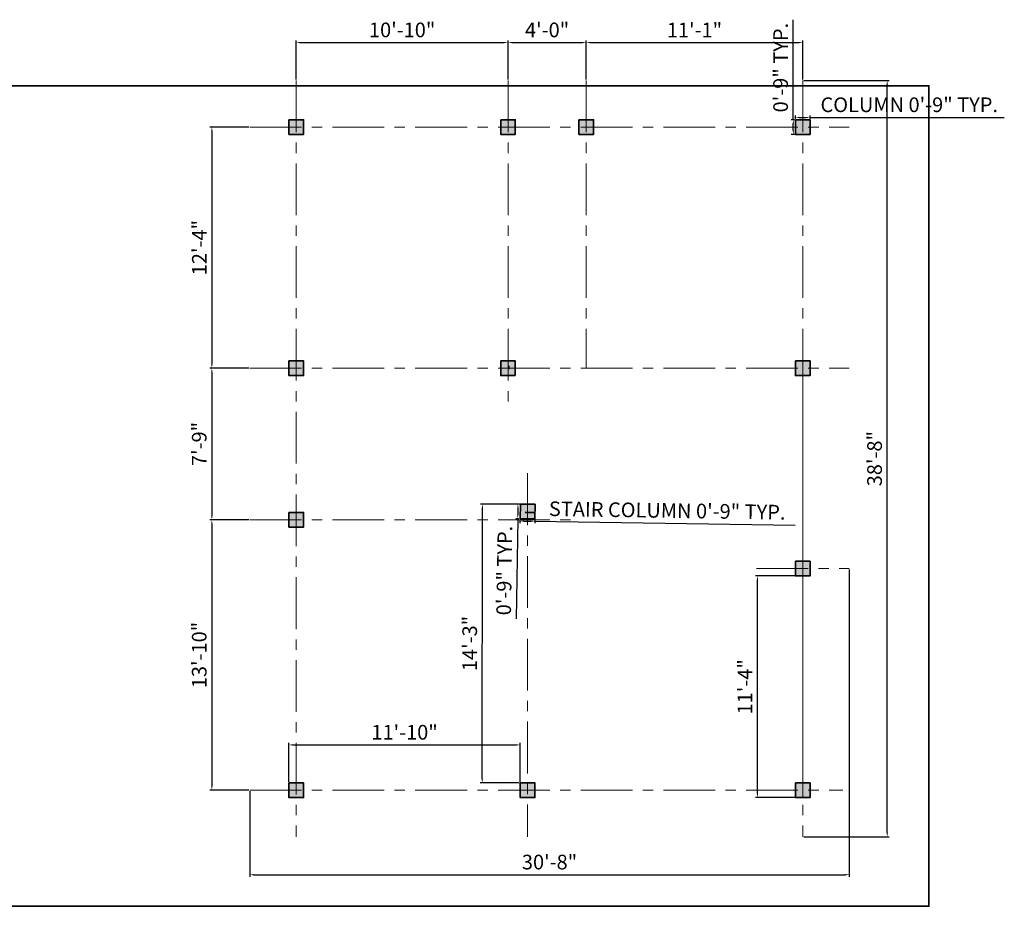
# Model space of a CAD drawing. Units: inches. Extents: x 2289 to 3796, y 1741 to 2286.
# Tile 4 of 4: x 3192 to 3796, y 1742 to 2286. Entities that reach past the tile are written whole.
import ezdxf

# ---------------------------------------------------------------- set-up
doc = ezdxf.new("R2010")
doc.units = ezdxf.units.IN
doc.linetypes.add('CENTER', pattern=[50.8, 31.75, -6.35, 6.35, -6.35])
for name, color, linetype, lineweight in [('A-ANNO-DIMS', 2, 'Continuous', 18), ('A-ANNO-TTLB', 7, 'Continuous', 35), ('S-COLS', 1, 'Continuous', 35), ('S-COLS-PATT', 1, 'Continuous', 13), ('S-GRID', 8, 'CENTER', 18)]:
    doc.layers.add(name, color=color, linetype=linetype, lineweight=lineweight)
doc.styles.get("Standard").update_dxf_attribs({"font": 'arial.ttf'})
doc.dimstyles.new('ISO-25', dxfattribs={"dimtxt": 9, "dimasz": 2.5, "dimexe": 1.25, "dimexo": 0.625, "dimgap": 2, "dimtad": 1, "dimdec": 1, "dimlunit": 4, "dimtxsty": 'Standard', "dimcen": 2.5, "dimadec": 0, "dimazin": 0, "dimtfac": 1, "dimtdec": 1, "dimtmove": 0, "dimatfit": 3, "dimfxl": 1, "dimarcsym": 0})

# ---------------------------------------------------------------- blocks, each defined once
blk = doc.blocks.new('COL-9X9')
h = blk.add_hatch(color=256)
h.dxf.hatch_style = 1
h.paths.add_polyline_path([(0, 9), (0, 0), (9, 0), (9, 9)])
blk.add_lwpolyline([(0, 9), (9, 9), (9, 0), (0, 0)], close=True)
blk = doc.blocks.new('COL-9X9-INT')
h = blk.add_hatch(color=256)
h.dxf.hatch_style = 1
h.paths.add_polyline_path([(9, 0), (9, 9), (0, 9), (0, 0)])
blk.add_lwpolyline([(0, 9), (9, 9), (9, 0), (0, 0)], close=True)
blk = doc.blocks.new('COL-9X9-STAIR')
h = blk.add_hatch(color=256)
h.dxf.hatch_style = 1
h.paths.add_polyline_path([(9, 0), (9, 9), (0, 9), (0, 0)])
blk.add_lwpolyline([(0.01, 9.14), (9.01, 9.14), (9.01, 0.14), (0.01, 0.14)], close=True)
blk = doc.blocks.new('*D23')
at = {"layer": 'A-ANNO-DIMS', "color": 0, "lineweight": -2, "transparency": 16777216}
for p, q in [((3668.24, 2225.01), (3668.24, 2226.99)), ((3670.74, 2225.74), (3674.74, 2225.74)), ((3677.24, 2225.01), (3677.24, 2226.99)), ((3677.24, 2225.74), (3796.47, 2225.74))]:
    blk.add_line(p, q, dxfattribs=at)
at = {"layer": 'A-ANNO-DIMS', "color": 0, "transparency": 16777216}
for points in [[(3670.74, 2226.15), (3670.74, 2225.32), (3668.24, 2225.74)], [(3674.74, 2226.15), (3674.74, 2225.32), (3677.24, 2225.74)]]:
    blk.add_solid(points, dxfattribs=at)
at = {"layer": 'Defpoints', "color": 0, "transparency": 16777216}
for p in [(3677.24, 2225.74), (3668.24, 2224.39), (3677.24, 2224.39)]:
    blk.add_point(p, dxfattribs=at)
at = {"layer": 'A-ANNO-DIMS', "color": 0, "transparency": 16777216, "insert": (3738.1, 2232.39), "char_height": 9, "attachment_point": 5}
blk.add_mtext('COLUMN 0\'-9" TYP.', dxfattribs=at)
blk = doc.blocks.new('*D24')
at = {"layer": 'A-ANNO-DIMS', "color": 0, "lineweight": -2, "transparency": 16777216}
for p, q in [((3666.89, 2224.39), (3666.89, 2285.75)), ((3667.61, 2224.39), (3665.64, 2224.39)), ((3666.89, 2217.89), (3666.89, 2221.89)), ((3667.61, 2215.39), (3665.64, 2215.39))]:
    blk.add_line(p, q, dxfattribs=at)
at = {"layer": 'A-ANNO-DIMS', "color": 0, "transparency": 16777216}
for points in [[(3666.47, 2221.89), (3667.3, 2221.89), (3666.89, 2224.39)], [(3666.47, 2217.89), (3667.3, 2217.89), (3666.89, 2215.39)]]:
    blk.add_solid(points, dxfattribs=at)
at = {"layer": 'Defpoints', "color": 0, "transparency": 16777216}
for p in [(3666.89, 2224.39), (3668.24, 2224.39), (3668.24, 2215.39)]:
    blk.add_point(p, dxfattribs=at)
at = {"layer": 'A-ANNO-DIMS', "color": 0, "transparency": 16777216, "insert": (3660.29, 2256.32), "char_height": 9, "attachment_point": 5, "rotation": 90}
blk.add_mtext('0\'-9" TYP.', dxfattribs=at)
blk = doc.blocks.new('*D27')
at = {"layer": 'A-ANNO-DIMS', "color": 0, "lineweight": -2, "transparency": 16777216}
for p, q in [((3499.08, 1978.87), (3499.05, 1976.87)), ((3501.56, 1978.09), (3505.7, 1978.02)), ((3508.21, 1978.73), (3508.18, 1976.73)), ((3508.2, 1977.98), (3668, 1975.53))]:
    blk.add_line(p, q, dxfattribs=at)
at = {"layer": 'A-ANNO-DIMS', "color": 0, "transparency": 16777216}
for points in [[(3501.57, 1978.5), (3501.56, 1977.67), (3499.07, 1978.12)], [(3505.71, 1978.44), (3505.7, 1977.61), (3508.2, 1977.98)]]:
    blk.add_solid(points, dxfattribs=at)
at = {"layer": 'Defpoints', "color": 0, "transparency": 16777216}
for p in [(3499.09, 1979.5), (3508.2, 1977.98), (3508.22, 1979.35)]:
    blk.add_point(p, dxfattribs=at)
at = {"layer": 'A-ANNO-DIMS', "color": 0, "transparency": 16777216, "insert": (3589.45, 1983.39), "char_height": 9, "attachment_point": 5, "rotation": 359.11913}
blk.add_mtext('STAIR COLUMN 0\'-9" TYP.', dxfattribs=at)
blk = doc.blocks.new('*D28')
at = {"layer": 'A-ANNO-DIMS', "color": 0, "lineweight": -2, "transparency": 16777216}
for p, q in [((3498.6, 1988.52), (3496.6, 1988.55)), ((3497.82, 1986.03), (3497.75, 1982.02)), ((3498.46, 1979.5), (3496.47, 1979.54)), ((3497.72, 1979.52), (3496.77, 1918.16))]:
    blk.add_line(p, q, dxfattribs=at)
at = {"layer": 'A-ANNO-DIMS', "color": 0, "transparency": 16777216}
for points in [[(3497.4, 1986.04), (3498.23, 1986.02), (3497.85, 1988.53)], [(3497.34, 1982.02), (3498.17, 1982.01), (3497.72, 1979.52)]]:
    blk.add_solid(points, dxfattribs=at)
at = {"layer": 'Defpoints', "color": 0, "transparency": 16777216}
for p in [(3499.22, 1988.51), (3497.72, 1979.52), (3499.09, 1979.5)]:
    blk.add_point(p, dxfattribs=at)
at = {"layer": 'A-ANNO-DIMS', "color": 0, "transparency": 16777216, "insert": (3490.63, 1947.69), "char_height": 9, "attachment_point": 5, "rotation": 89.11913}
blk.add_mtext('0\'-9" TYP.', dxfattribs=at)
blk = doc.blocks.new('*D64')
at = {"layer": 'A-ANNO-DIMS', "color": 0, "lineweight": -2, "transparency": 16777216}
for p, q in [((3701.24, 1948.26), (3701.24, 1759.81)), ((3333.24, 1812.26), (3333.24, 1759.81)), ((3335.74, 1761.06), (3698.74, 1761.06))]:
    blk.add_line(p, q, dxfattribs=at)
at = {"layer": 'A-ANNO-DIMS', "color": 0, "transparency": 16777216}
for points in [[(3335.74, 1761.48), (3335.74, 1760.64), (3333.24, 1761.06)], [(3698.74, 1761.48), (3698.74, 1760.64), (3701.24, 1761.06)]]:
    blk.add_solid(points, dxfattribs=at)
at = {"layer": 'Defpoints', "color": 0, "transparency": 16777216}
for p in [(3701.24, 1948.89), (3333.24, 1812.89), (3701.24, 1761.06)]:
    blk.add_point(p, dxfattribs=at)
at = {"layer": 'A-ANNO-DIMS', "color": 0, "transparency": 16777216, "insert": (3517.24, 1767.66), "char_height": 9, "attachment_point": 5}
blk.add_mtext('30\'-8"', dxfattribs=at)
blk = doc.blocks.new('*D65')
at = {"layer": 'A-ANNO-DIMS', "color": 0, "lineweight": -2, "transparency": 16777216}
for p, q in [((3673.36, 2248.39), (3725.81, 2248.39)), ((3724.56, 1786.89), (3724.56, 2245.89)), ((3673.36, 1784.39), (3725.81, 1784.39))]:
    blk.add_line(p, q, dxfattribs=at)
at = {"layer": 'A-ANNO-DIMS', "color": 0, "transparency": 16777216}
for points in [[(3724.14, 2245.89), (3724.98, 2245.89), (3724.56, 2248.39)], [(3724.14, 1786.89), (3724.98, 1786.89), (3724.56, 1784.39)]]:
    blk.add_solid(points, dxfattribs=at)
at = {"layer": 'Defpoints', "color": 0, "transparency": 16777216}
for p in [(3672.74, 2248.39), (3724.56, 2248.39), (3672.74, 1784.39)]:
    blk.add_point(p, dxfattribs=at)
at = {"layer": 'A-ANNO-DIMS', "color": 0, "transparency": 16777216, "insert": (3717.96, 2016.39), "char_height": 9, "attachment_point": 5, "rotation": 90}
blk.add_mtext('38\'-8"', dxfattribs=at)
blk = doc.blocks.new('*D66')
at = {"layer": 'A-ANNO-DIMS', "color": 0, "lineweight": -2, "transparency": 16777216}
for p, q in [((3361.74, 2249.01), (3361.74, 2272.96)), ((3364.24, 2271.71), (3489.24, 2271.71)), ((3491.74, 2249.01), (3491.74, 2272.96))]:
    blk.add_line(p, q, dxfattribs=at)
at = {"layer": 'A-ANNO-DIMS', "color": 0, "transparency": 16777216}
for points in [[(3364.24, 2272.13), (3364.24, 2271.29), (3361.74, 2271.71)], [(3489.24, 2272.13), (3489.24, 2271.29), (3491.74, 2271.71)]]:
    blk.add_solid(points, dxfattribs=at)
at = {"layer": 'Defpoints', "color": 0, "transparency": 16777216}
for p in [(3491.74, 2271.71), (3361.74, 2248.39), (3491.74, 2248.39)]:
    blk.add_point(p, dxfattribs=at)
at = {"layer": 'A-ANNO-DIMS', "color": 0, "transparency": 16777216, "insert": (3426.74, 2278.31), "char_height": 9, "attachment_point": 5}
blk.add_mtext('10\'-10"', dxfattribs=at)
blk = doc.blocks.new('*D67')
at = {"layer": 'A-ANNO-DIMS', "color": 0, "lineweight": -2, "transparency": 16777216}
for p, q in [((3491.74, 2249.01), (3491.74, 2272.96)), ((3494.24, 2271.71), (3537.24, 2271.71)), ((3539.74, 2249.01), (3539.74, 2272.96))]:
    blk.add_line(p, q, dxfattribs=at)
at = {"layer": 'A-ANNO-DIMS', "color": 0, "transparency": 16777216}
for points in [[(3494.24, 2272.13), (3494.24, 2271.29), (3491.74, 2271.71)], [(3537.24, 2272.13), (3537.24, 2271.29), (3539.74, 2271.71)]]:
    blk.add_solid(points, dxfattribs=at)
at = {"layer": 'Defpoints', "color": 0, "transparency": 16777216}
for p in [(3539.74, 2271.71), (3491.74, 2248.39), (3539.74, 2248.39)]:
    blk.add_point(p, dxfattribs=at)
at = {"layer": 'A-ANNO-DIMS', "color": 0, "transparency": 16777216, "insert": (3515.74, 2278.31), "char_height": 9, "attachment_point": 5}
blk.add_mtext('4\'-0"', dxfattribs=at)
blk = doc.blocks.new('*D68')
at = {"layer": 'A-ANNO-DIMS', "color": 0, "lineweight": -2, "transparency": 16777216}
for p, q in [((3539.74, 2249.01), (3539.74, 2272.96)), ((3542.24, 2271.71), (3670.24, 2271.71)), ((3672.74, 2249.01), (3672.74, 2272.96))]:
    blk.add_line(p, q, dxfattribs=at)
at = {"layer": 'A-ANNO-DIMS', "color": 0, "transparency": 16777216}
for points in [[(3542.24, 2272.13), (3542.24, 2271.29), (3539.74, 2271.71)], [(3670.24, 2272.13), (3670.24, 2271.29), (3672.74, 2271.71)]]:
    blk.add_solid(points, dxfattribs=at)
at = {"layer": 'Defpoints', "color": 0, "transparency": 16777216}
for p in [(3672.74, 2271.71), (3539.74, 2248.39), (3672.74, 2248.39)]:
    blk.add_point(p, dxfattribs=at)
at = {"layer": 'A-ANNO-DIMS', "color": 0, "transparency": 16777216, "insert": (3606.24, 2278.23), "char_height": 9, "attachment_point": 5}
blk.add_mtext('11\'-1"', dxfattribs=at)
blk = doc.blocks.new('*D69')
at = {"layer": 'A-ANNO-DIMS', "color": 0, "lineweight": -2, "transparency": 16777216}
for p, q in [((3357.24, 1818.01), (3357.24, 1841.96)), ((3359.74, 1840.71), (3496.74, 1840.71)), ((3499.24, 1818.01), (3499.24, 1841.96))]:
    blk.add_line(p, q, dxfattribs=at)
at = {"layer": 'A-ANNO-DIMS', "color": 0, "transparency": 16777216}
for points in [[(3359.74, 1841.13), (3359.74, 1840.29), (3357.24, 1840.71)], [(3496.74, 1841.13), (3496.74, 1840.29), (3499.24, 1840.71)]]:
    blk.add_solid(points, dxfattribs=at)
at = {"layer": 'Defpoints', "color": 0, "transparency": 16777216}
for p in [(3499.24, 1840.71), (3357.24, 1817.39), (3499.24, 1817.39)]:
    blk.add_point(p, dxfattribs=at)
at = {"layer": 'A-ANNO-DIMS', "color": 0, "transparency": 16777216, "insert": (3428.24, 1847.31), "char_height": 9, "attachment_point": 5}
blk.add_mtext('11\'-10"', dxfattribs=at)
blk = doc.blocks.new('*D70')
at = {"layer": 'A-ANNO-DIMS', "color": 0, "lineweight": -2, "transparency": 16777216}
for p, q in [((3332.61, 2219.89), (3308.66, 2219.89)), ((3309.91, 2217.39), (3309.91, 2074.39)), ((3332.61, 2071.89), (3308.66, 2071.89))]:
    blk.add_line(p, q, dxfattribs=at)
at = {"layer": 'A-ANNO-DIMS', "color": 0, "transparency": 16777216}
for points in [[(3309.49, 2217.39), (3310.33, 2217.39), (3309.91, 2219.89)], [(3309.49, 2074.39), (3310.33, 2074.39), (3309.91, 2071.89)]]:
    blk.add_solid(points, dxfattribs=at)
at = {"layer": 'Defpoints', "color": 0, "transparency": 16777216}
for p in [(3333.24, 2219.89), (3309.91, 2071.89), (3333.24, 2071.89)]:
    blk.add_point(p, dxfattribs=at)
at = {"layer": 'A-ANNO-DIMS', "color": 0, "transparency": 16777216, "insert": (3303.39, 2145.89), "char_height": 9, "attachment_point": 5, "rotation": 90}
blk.add_mtext('12\'-4"', dxfattribs=at)
blk = doc.blocks.new('*D71')
at = {"layer": 'A-ANNO-DIMS', "color": 0, "lineweight": -2, "transparency": 16777216}
for p, q in [((3332.61, 2071.89), (3308.66, 2071.89)), ((3309.91, 2069.39), (3309.91, 1981.39)), ((3332.61, 1978.89), (3308.66, 1978.89))]:
    blk.add_line(p, q, dxfattribs=at)
at = {"layer": 'A-ANNO-DIMS', "color": 0, "transparency": 16777216}
for points in [[(3309.49, 2069.39), (3310.33, 2069.39), (3309.91, 2071.89)], [(3309.49, 1981.39), (3310.33, 1981.39), (3309.91, 1978.89)]]:
    blk.add_solid(points, dxfattribs=at)
at = {"layer": 'Defpoints', "color": 0, "transparency": 16777216}
for p in [(3333.24, 2071.89), (3309.91, 1978.89), (3333.24, 1978.89)]:
    blk.add_point(p, dxfattribs=at)
at = {"layer": 'A-ANNO-DIMS', "color": 0, "transparency": 16777216, "insert": (3303.32, 2025.39), "char_height": 9, "attachment_point": 5, "rotation": 90}
blk.add_mtext('7\'-9"', dxfattribs=at)
blk = doc.blocks.new('*D72')
at = {"layer": 'A-ANNO-DIMS', "color": 0, "lineweight": -2, "transparency": 16777216}
for p, q in [((3332.61, 1978.89), (3308.66, 1978.89)), ((3309.91, 1976.39), (3309.91, 1815.39)), ((3332.61, 1812.89), (3308.66, 1812.89))]:
    blk.add_line(p, q, dxfattribs=at)
at = {"layer": 'A-ANNO-DIMS', "color": 0, "transparency": 16777216}
for points in [[(3309.49, 1976.39), (3310.33, 1976.39), (3309.91, 1978.89)], [(3309.49, 1815.39), (3310.33, 1815.39), (3309.91, 1812.89)]]:
    blk.add_solid(points, dxfattribs=at)
at = {"layer": 'Defpoints', "color": 0, "transparency": 16777216}
for p in [(3333.24, 1978.89), (3309.91, 1812.89), (3333.24, 1812.89)]:
    blk.add_point(p, dxfattribs=at)
at = {"layer": 'A-ANNO-DIMS', "color": 0, "transparency": 16777216, "insert": (3303.31, 1895.89), "char_height": 9, "attachment_point": 5, "rotation": 90}
blk.add_mtext('13\'-10"', dxfattribs=at)
blk = doc.blocks.new('*D73')
at = {"layer": 'A-ANNO-DIMS', "color": 0, "lineweight": -2, "transparency": 16777216}
for p, q in [((3667.61, 1944.39), (3643.66, 1944.39)), ((3644.91, 1810.89), (3644.91, 1941.89)), ((3667.61, 1808.39), (3643.66, 1808.39))]:
    blk.add_line(p, q, dxfattribs=at)
at = {"layer": 'A-ANNO-DIMS', "color": 0, "transparency": 16777216}
for points in [[(3644.49, 1941.89), (3645.33, 1941.89), (3644.91, 1944.39)], [(3644.49, 1810.89), (3645.33, 1810.89), (3644.91, 1808.39)]]:
    blk.add_solid(points, dxfattribs=at)
at = {"layer": 'Defpoints', "color": 0, "transparency": 16777216}
for p in [(3644.91, 1944.39), (3668.24, 1944.39), (3668.24, 1808.39)]:
    blk.add_point(p, dxfattribs=at)
at = {"layer": 'A-ANNO-DIMS', "color": 0, "transparency": 16777216, "insert": (3638.39, 1876.39), "char_height": 9, "attachment_point": 5, "rotation": 90}
blk.add_mtext('11\'-4"', dxfattribs=at)
blk = doc.blocks.new('*D74')
at = {"layer": 'A-ANNO-DIMS', "color": 0, "lineweight": -2, "transparency": 16777216}
for p, q in [((3498.74, 1988.49), (3474.79, 1988.51)), ((3475.91, 1819.9), (3476.04, 1986.01)), ((3498.61, 1817.39), (3474.66, 1817.4))]:
    blk.add_line(p, q, dxfattribs=at)
at = {"layer": 'A-ANNO-DIMS', "color": 0, "transparency": 16777216}
for points in [[(3475.62, 1986.01), (3476.45, 1986.01), (3476.04, 1988.51)], [(3475.5, 1819.9), (3476.33, 1819.9), (3475.91, 1817.4)]]:
    blk.add_solid(points, dxfattribs=at)
at = {"layer": 'Defpoints', "color": 0, "transparency": 16777216}
for p in [(3476.04, 1988.51), (3499.36, 1988.49), (3499.24, 1817.39)]:
    blk.add_point(p, dxfattribs=at)
at = {"layer": 'A-ANNO-DIMS', "color": 0, "transparency": 16777216, "insert": (3469.38, 1902.96), "char_height": 9, "attachment_point": 5, "rotation": 89.95719}
blk.add_mtext('14\'-3"', dxfattribs=at)

msp = doc.modelspace()

# ---------------------------------------------------------------- hatches: boundary and pattern name
at = {"layer": 'S-COLS-PATT'}
h = msp.add_hatch(color=256, dxfattribs=at)
h.dxf.hatch_style = 1
h.paths.add_polyline_path([(3668.29, 1953.41), (3668.29, 1944.41), (3677.29, 1944.41), (3677.29, 1953.41)])

# ---------------------------------------------------------------- linework, layer by layer
at = {"layer": 'A-ANNO-TTLB'}
msp.add_lwpolyline([(2318.16, 2245.19), (3750.19, 2245.19), (3750.19, 1741.69), (2318.16, 1741.69)], close=True, dxfattribs=at)
at = {"layer": 'S-COLS'}
for p, q in [((3492.24, 2073.39), (3492.24, 2071.39)), ((3496.24, 2073.39), (3496.24, 2067.39)), ((3502.24, 1983.39), (3504.24, 1983.39)), ((3504.24, 1983.39), (3508.24, 1983.39)), ((3504.24, 1979.39), (3508.24, 1979.39)), ((3499.24, 1817.39), (3499.24, 1808.39)), ((3668.24, 1817.39), (3677.24, 1817.39))]:
    msp.add_line(p, q, dxfattribs=at)
msp.add_lwpolyline([(3668.24, 1953.39), (3677.24, 1953.39), (3677.24, 1944.39), (3668.24, 1944.39)], close=True, dxfattribs=at)
at = {"layer": 'S-GRID'}
for p, q in [((3361.74, 2248.39), (3361.74, 1784.39)), ((3491.74, 2248.39), (3491.74, 2047.39)), ((3539.74, 2248.39), (3539.74, 2071.89)), ((3672.74, 2248.39), (3672.74, 1784.39)), ((3333.24, 2219.89), (3701.24, 2219.89)), ((3672.74, 2076.39), (3672.74, 1808.39)), ((3333.24, 2071.89), (3701.24, 2071.89)), ((3503.74, 2007.39), (3503.74, 1784.39)), ((3333.24, 1978.89), (3532.23, 1978.89)), ((3644.24, 1948.89), (3701.24, 1948.89)), ((3333.24, 1812.89), (3697.24, 1812.89))]:
    msp.add_line(p, q, dxfattribs=at)

# ---------------------------------------------------------------- block references
at = {"layer": 'S-COLS'}
for p in [(3357.24, 2215.39), (3487.24, 2215.39), (3535.24, 2215.39), (3668.24, 2215.39), (3357.24, 2067.39), (3668.24, 2067.39), (3357.24, 1974.39), (3357.24, 1808.39), (3499.24, 1808.39), (3668.24, 1808.39)]:
    msp.add_blockref('COL-9X9', p, dxfattribs=at)
for name, p, rotation in [('COL-9X9-INT', (3496.24, 2076.39), 180), ('COL-9X9-STAIR', (3499.22, 1988.51), 269.1191340703009)]:
    msp.add_blockref(name, p, dxfattribs=dict(at, rotation=rotation))

# ---------------------------------------------------------------- dimensions: what is measured, and where the dimension line sits
at = {"layer": 'A-ANNO-DIMS'}
for base, p1, p2, angle, text, picture, middle in [((3666.89, 2224.39), (3668.24, 2215.39), (3668.24, 2224.39), 90, '<> TYP.', '*D24', (3660.29, 2256.32)), ((3508.2, 1977.98), (3499.09, 1979.5), (3508.22, 1979.35), 359.11913, 'STAIR COLUMN <> TYP.', '*D27', (3589.45, 1983.39)), ((3497.72, 1979.52), (3499.22, 1988.51), (3499.09, 1979.5), 269.11913, '<> TYP.', '*D28', (3490.63, 1947.69))]:
    dim = msp.add_linear_dim(base=base, p1=p1, p2=p2, angle=angle, text=text, dimstyle='ISO-25', override={"dimdec": 1, "dimlfac": 1, "dimrnd": 0, "dimzin": 1, "dimdsep": 46, "dimlunit": 4, "dimfrac": 2}, dxfattribs=at)
    dim.commit()
    dim.dimension.update_dxf_attribs({"geometry": picture, "text_midpoint": middle})
for base, p1, p2, picture, middle in [((3491.74, 2271.71), (3361.74, 2248.39), (3491.74, 2248.39), '*D66', (3426.74, 2278.31)), ((3539.74, 2271.71), (3491.74, 2248.39), (3539.74, 2248.39), '*D67', (3515.74, 2278.31)), ((3672.74, 2271.71), (3539.74, 2248.39), (3672.74, 2248.39), '*D68', (3606.24, 2278.23)), ((3701.24, 1761.06), (3333.24, 1812.89), (3701.24, 1948.89), '*D64', (3517.24, 1767.66)), ((3499.24, 1840.71), (3357.24, 1817.39), (3499.24, 1817.39), '*D69', (3428.24, 1847.31))]:
    dim = msp.add_linear_dim(base=base, p1=p1, p2=p2, dimstyle='ISO-25', override={"dimdec": 1, "dimlfac": 1, "dimrnd": 0, "dimzin": 1, "dimdsep": 46, "dimlunit": 4, "dimfrac": 2}, dxfattribs=at)
    dim.commit()
    dim.dimension.update_dxf_attribs({"geometry": picture, "text_midpoint": middle})
dim = msp.add_linear_dim(base=(3677.24, 2225.74), p1=(3668.24, 2224.39), p2=(3677.24, 2224.39), text='COLUMN <> TYP.', dimstyle='ISO-25', override={"dimdec": 1, "dimlfac": 1, "dimrnd": 0, "dimzin": 1, "dimdsep": 46, "dimlunit": 4, "dimfrac": 2}, dxfattribs=at)
dim.commit()
dim.dimension.update_dxf_attribs({"geometry": '*D23', "text_midpoint": (3738.1, 2232.39)})
for base, p1, p2, angle, picture, middle in [((3724.56, 2248.39), (3672.74, 1784.39), (3672.74, 2248.39), 90, '*D65', (3717.96, 2016.39)), ((3309.91, 2071.89), (3333.24, 2219.89), (3333.24, 2071.89), 90, '*D70', (3303.39, 2145.89)), ((3309.91, 1978.89), (3333.24, 2071.89), (3333.24, 1978.89), 90, '*D71', (3303.32, 2025.39)), ((3476.04, 1988.51), (3499.24, 1817.39), (3499.36, 1988.49), 89.95719, '*D74', (3469.38, 1902.96)), ((3309.91, 1812.89), (3333.24, 1978.89), (3333.24, 1812.89), 90, '*D72', (3303.31, 1895.89)), ((3644.91, 1944.39), (3668.24, 1808.39), (3668.24, 1944.39), 90, '*D73', (3638.39, 1876.39))]:
    dim = msp.add_linear_dim(base=base, p1=p1, p2=p2, angle=angle, dimstyle='ISO-25', override={"dimdec": 1, "dimlfac": 1, "dimrnd": 0, "dimzin": 1, "dimdsep": 46, "dimlunit": 4, "dimfrac": 2}, dxfattribs=at)
    dim.commit()
    dim.dimension.update_dxf_attribs({"geometry": picture, "text_midpoint": middle})

doc.saveas('drawing.dxf')
